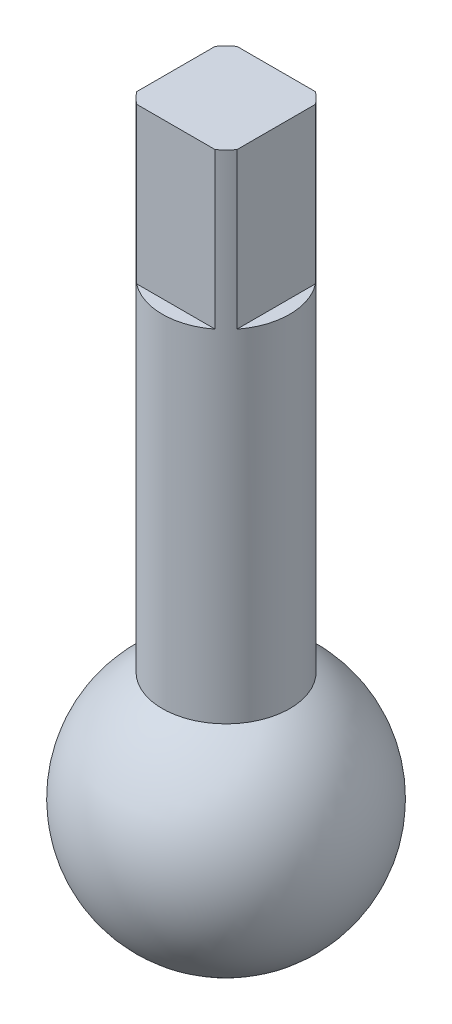
ISO-10303-21;
HEADER;
FILE_DESCRIPTION(('STEP AP214'),'2;1');
FILE_NAME('part.step','',(''),(''),'','','');
FILE_SCHEMA(('AUTOMOTIVE_DESIGN { 1 0 10303 214 1 1 1 1 }'));
ENDSEC;
DATA;
#1=APPLICATION_CONTEXT('core data for automotive mechanical design processes');
#2=APPLICATION_PROTOCOL_DEFINITION('international standard','automotive_design',2000,#1);
#3=PRODUCT_CONTEXT('',#1,'mechanical');
#4=PRODUCT('Part','Part','',(#3));
#5=PRODUCT_RELATED_PRODUCT_CATEGORY('part','',(#4));
#6=PRODUCT_DEFINITION_FORMATION('','',#4);
#7=PRODUCT_DEFINITION_CONTEXT('part definition',#1,'design');
#8=PRODUCT_DEFINITION('design','',#6,#7);
#9=PRODUCT_DEFINITION_SHAPE('','',#8);
#10=(LENGTH_UNIT() NAMED_UNIT(*) SI_UNIT(.MILLI.,.METRE.));
#11=(NAMED_UNIT(*) PLANE_ANGLE_UNIT() SI_UNIT($,.RADIAN.));
#12=(NAMED_UNIT(*) SI_UNIT($,.STERADIAN.) SOLID_ANGLE_UNIT());
#13=UNCERTAINTY_MEASURE_WITH_UNIT(LENGTH_MEASURE(1.E-05),#10,'distance_accuracy_value','');
#14=(GEOMETRIC_REPRESENTATION_CONTEXT(3) GLOBAL_UNCERTAINTY_ASSIGNED_CONTEXT((#13)) GLOBAL_UNIT_ASSIGNED_CONTEXT((#10,
#11,#12)) REPRESENTATION_CONTEXT('',''));
#15=CARTESIAN_POINT('',(0.,0.,0.));
#16=DIRECTION('',(0.,0.,1.));
#17=DIRECTION('',(1.,0.,0.));
#18=AXIS2_PLACEMENT_3D('',#15,#16,#17);
#19=CARTESIAN_POINT('',(0.,90.3,0.));
#20=DIRECTION('',(0.,-1.,0.));
#21=DIRECTION('',(0.,0.,-1.));
#22=AXIS2_PLACEMENT_3D('',#19,#20,#21);
#23=CYLINDRICAL_SURFACE('',#22,12.7);
#24=CARTESIAN_POINT('',(0.,-8.78850096542744,0.));
#25=DIRECTION('',(0.,-1.,0.));
#26=DIRECTION('',(0.,0.,-1.));
#27=AXIS2_PLACEMENT_3D('',#24,#25,#26);
#28=CIRCLE('',#27,12.7);
#29=CARTESIAN_POINT('',(0.,-8.78850096542744,-12.7));
#30=VERTEX_POINT('',#29);
#31=EDGE_CURVE('E11',#30,#30,#28,.T.);
#32=ORIENTED_EDGE('',*,*,#31,.F.);
#33=EDGE_LOOP('',(#32));
#34=FACE_BOUND('',#33,.T.);
#35=DIRECTION('',(0.,1.,0.));
#36=VECTOR('',#35,1.);
#37=CARTESIAN_POINT('',(-7.82879301041993,59.3,10.));
#38=LINE('',#37,#36);
#39=CARTESIAN_POINT('',(-7.82879301041993,59.3,10.));
#40=VERTEX_POINT('',#39);
#41=CARTESIAN_POINT('',(-7.82879301041993,90.3,10.));
#42=VERTEX_POINT('',#41);
#43=EDGE_CURVE('E102',#40,#42,#38,.T.);
#44=ORIENTED_EDGE('',*,*,#43,.T.);
#45=CARTESIAN_POINT('',(0.,90.3,0.));
#46=DIRECTION('',(0.,1.,0.));
#47=DIRECTION('',(0.,0.,1.));
#48=AXIS2_PLACEMENT_3D('',#45,#46,#47);
#49=CIRCLE('',#48,12.7);
#50=CARTESIAN_POINT('',(-10.,90.3,7.82879301041993));
#51=VERTEX_POINT('',#50);
#52=EDGE_CURVE('E130',#51,#42,#49,.T.);
#53=ORIENTED_EDGE('',*,*,#52,.F.);
#54=DIRECTION('',(0.,1.,0.));
#55=VECTOR('',#54,1.);
#56=CARTESIAN_POINT('',(-10.,59.3,7.82879301041993));
#57=LINE('',#56,#55);
#58=CARTESIAN_POINT('',(-10.,59.3,7.82879301041993));
#59=VERTEX_POINT('',#58);
#60=EDGE_CURVE('E57',#59,#51,#57,.T.);
#61=ORIENTED_EDGE('',*,*,#60,.F.);
#62=CARTESIAN_POINT('',(0.,59.3,0.));
#63=DIRECTION('',(0.,1.,0.));
#64=DIRECTION('',(0.,0.,1.));
#65=AXIS2_PLACEMENT_3D('',#62,#63,#64);
#66=CIRCLE('',#65,12.7);
#67=CARTESIAN_POINT('',(-10.,59.3,-7.82879301041993));
#68=VERTEX_POINT('',#67);
#69=EDGE_CURVE('E132',#68,#59,#66,.T.);
#70=ORIENTED_EDGE('',*,*,#69,.F.);
#71=DIRECTION('',(0.,1.,0.));
#72=VECTOR('',#71,1.);
#73=CARTESIAN_POINT('',(-10.,59.3,-7.82879301041993));
#74=LINE('',#73,#72);
#75=CARTESIAN_POINT('',(-10.,90.3,-7.82879301041993));
#76=VERTEX_POINT('',#75);
#77=EDGE_CURVE('E131',#68,#76,#74,.T.);
#78=ORIENTED_EDGE('',*,*,#77,.T.);
#79=CARTESIAN_POINT('',(-7.82879301041993,90.3,-10.));
#80=VERTEX_POINT('',#79);
#81=EDGE_CURVE('E170',#80,#76,#49,.T.);
#82=ORIENTED_EDGE('',*,*,#81,.F.);
#83=DIRECTION('',(0.,1.,0.));
#84=VECTOR('',#83,1.);
#85=CARTESIAN_POINT('',(-7.82879301041993,59.3,-10.));
#86=LINE('',#85,#84);
#87=CARTESIAN_POINT('',(-7.82879301041993,59.3,-10.));
#88=VERTEX_POINT('',#87);
#89=EDGE_CURVE('E61',#88,#80,#86,.T.);
#90=ORIENTED_EDGE('',*,*,#89,.F.);
#91=CARTESIAN_POINT('',(0.,59.3,0.));
#92=DIRECTION('',(0.,1.,0.));
#93=DIRECTION('',(0.,0.,1.));
#94=AXIS2_PLACEMENT_3D('',#91,#92,#93);
#95=CIRCLE('',#94,12.7);
#96=CARTESIAN_POINT('',(7.82879301041993,59.3,-10.));
#97=VERTEX_POINT('',#96);
#98=EDGE_CURVE('E145',#97,#88,#95,.T.);
#99=ORIENTED_EDGE('',*,*,#98,.F.);
#100=DIRECTION('',(0.,1.,0.));
#101=VECTOR('',#100,1.);
#102=CARTESIAN_POINT('',(7.82879301041993,59.3,-10.));
#103=LINE('',#102,#101);
#104=CARTESIAN_POINT('',(7.82879301041993,90.3,-10.));
#105=VERTEX_POINT('',#104);
#106=EDGE_CURVE('E147',#97,#105,#103,.T.);
#107=ORIENTED_EDGE('',*,*,#106,.T.);
#108=CARTESIAN_POINT('',(10.,90.3,-7.82879301041993));
#109=VERTEX_POINT('',#108);
#110=EDGE_CURVE('E165',#109,#105,#49,.T.);
#111=ORIENTED_EDGE('',*,*,#110,.F.);
#112=DIRECTION('',(0.,1.,0.));
#113=VECTOR('',#112,1.);
#114=CARTESIAN_POINT('',(10.,59.3,-7.82879301041993));
#115=LINE('',#114,#113);
#116=CARTESIAN_POINT('',(10.,59.3,-7.82879301041993));
#117=VERTEX_POINT('',#116);
#118=EDGE_CURVE('E149',#117,#109,#115,.T.);
#119=ORIENTED_EDGE('',*,*,#118,.F.);
#120=CARTESIAN_POINT('',(0.,59.3,0.));
#121=DIRECTION('',(0.,1.,0.));
#122=DIRECTION('',(0.,0.,1.));
#123=AXIS2_PLACEMENT_3D('',#120,#121,#122);
#124=CIRCLE('',#123,12.7);
#125=CARTESIAN_POINT('',(10.,59.3,7.82879301041993));
#126=VERTEX_POINT('',#125);
#127=EDGE_CURVE('E154',#126,#117,#124,.T.);
#128=ORIENTED_EDGE('',*,*,#127,.F.);
#129=DIRECTION('',(0.,1.,0.));
#130=VECTOR('',#129,1.);
#131=CARTESIAN_POINT('',(10.,59.3,7.82879301041993));
#132=LINE('',#131,#130);
#133=CARTESIAN_POINT('',(10.,90.3,7.82879301041993));
#134=VERTEX_POINT('',#133);
#135=EDGE_CURVE('E157',#126,#134,#132,.T.);
#136=ORIENTED_EDGE('',*,*,#135,.T.);
#137=CARTESIAN_POINT('',(7.82879301041993,90.3,10.));
#138=VERTEX_POINT('',#137);
#139=EDGE_CURVE('E47',#138,#134,#49,.T.);
#140=ORIENTED_EDGE('',*,*,#139,.F.);
#141=DIRECTION('',(0.,1.,0.));
#142=VECTOR('',#141,1.);
#143=CARTESIAN_POINT('',(7.82879301041993,59.3,10.));
#144=LINE('',#143,#142);
#145=CARTESIAN_POINT('',(7.82879301041993,59.3,10.));
#146=VERTEX_POINT('',#145);
#147=EDGE_CURVE('E116',#146,#138,#144,.T.);
#148=ORIENTED_EDGE('',*,*,#147,.F.);
#149=CARTESIAN_POINT('',(0.,59.3,0.));
#150=DIRECTION('',(0.,1.,0.));
#151=DIRECTION('',(0.,0.,1.));
#152=AXIS2_PLACEMENT_3D('',#149,#150,#151);
#153=CIRCLE('',#152,12.7);
#154=EDGE_CURVE('E120',#40,#146,#153,.T.);
#155=ORIENTED_EDGE('',*,*,#154,.F.);
#156=EDGE_LOOP('',(#44,#53,#61,#70,#78,#82,#90,#99,#107,#111,#119,#128,#136,#140,#148,#155));
#157=FACE_BOUND('',#156,.T.);
#158=ADVANCED_FACE('F41',(#34,#157),#23,.T.);
#159=CARTESIAN_POINT('',(0.,90.3,0.));
#160=DIRECTION('',(0.,1.,0.));
#161=DIRECTION('',(0.,0.,1.));
#162=AXIS2_PLACEMENT_3D('',#159,#160,#161);
#163=PLANE('',#162);
#164=ORIENTED_EDGE('',*,*,#52,.T.);
#165=DIRECTION('',(1.,0.,0.));
#166=VECTOR('',#165,1.);
#167=CARTESIAN_POINT('',(0.,90.3,10.));
#168=LINE('',#167,#166);
#169=EDGE_CURVE('E111',#42,#138,#168,.T.);
#170=ORIENTED_EDGE('',*,*,#169,.T.);
#171=ORIENTED_EDGE('',*,*,#139,.T.);
#172=DIRECTION('',(0.,0.,-1.));
#173=VECTOR('',#172,1.);
#174=CARTESIAN_POINT('',(10.,90.3,0.));
#175=LINE('',#174,#173);
#176=EDGE_CURVE('E151',#134,#109,#175,.T.);
#177=ORIENTED_EDGE('',*,*,#176,.T.);
#178=ORIENTED_EDGE('',*,*,#110,.T.);
#179=DIRECTION('',(-1.,0.,0.));
#180=VECTOR('',#179,1.);
#181=CARTESIAN_POINT('',(0.,90.3,-10.));
#182=LINE('',#181,#180);
#183=EDGE_CURVE('E141',#105,#80,#182,.T.);
#184=ORIENTED_EDGE('',*,*,#183,.T.);
#185=ORIENTED_EDGE('',*,*,#81,.T.);
#186=DIRECTION('',(0.,0.,1.));
#187=VECTOR('',#186,1.);
#188=CARTESIAN_POINT('',(-10.,90.3,0.));
#189=LINE('',#188,#187);
#190=EDGE_CURVE('E135',#76,#51,#189,.T.);
#191=ORIENTED_EDGE('',*,*,#190,.T.);
#192=EDGE_LOOP('',(#164,#170,#171,#177,#178,#184,#185,#191));
#193=FACE_BOUND('',#192,.T.);
#194=ADVANCED_FACE('F167',(#193),#163,.T.);
#195=CARTESIAN_POINT('',(10.,59.3,0.));
#196=DIRECTION('',(1.,0.,0.));
#197=DIRECTION('',(0.,0.,-1.));
#198=AXIS2_PLACEMENT_3D('',#195,#196,#197);
#199=PLANE('',#198);
#200=ORIENTED_EDGE('',*,*,#176,.F.);
#201=ORIENTED_EDGE('',*,*,#135,.F.);
#202=DIRECTION('',(0.,0.,-1.));
#203=VECTOR('',#202,1.);
#204=CARTESIAN_POINT('',(10.,59.3,0.));
#205=LINE('',#204,#203);
#206=EDGE_CURVE('E155',#126,#117,#205,.T.);
#207=ORIENTED_EDGE('',*,*,#206,.T.);
#208=ORIENTED_EDGE('',*,*,#118,.T.);
#209=EDGE_LOOP('',(#200,#201,#207,#208));
#210=FACE_BOUND('',#209,.T.);
#211=ADVANCED_FACE('F186',(#210),#199,.T.);
#212=CARTESIAN_POINT('',(0.,59.3,0.));
#213=DIRECTION('',(0.,1.,0.));
#214=DIRECTION('',(0.,0.,1.));
#215=AXIS2_PLACEMENT_3D('',#212,#213,#214);
#216=PLANE('',#215);
#217=ORIENTED_EDGE('',*,*,#206,.F.);
#218=ORIENTED_EDGE('',*,*,#127,.T.);
#219=EDGE_LOOP('',(#217,#218));
#220=FACE_BOUND('',#219,.T.);
#221=ADVANCED_FACE('F193',(#220),#216,.T.);
#222=CARTESIAN_POINT('',(0.,59.3,-10.));
#223=DIRECTION('',(0.,0.,-1.));
#224=DIRECTION('',(-1.,0.,0.));
#225=AXIS2_PLACEMENT_3D('',#222,#223,#224);
#226=PLANE('',#225);
#227=ORIENTED_EDGE('',*,*,#183,.F.);
#228=ORIENTED_EDGE('',*,*,#106,.F.);
#229=DIRECTION('',(-1.,0.,0.));
#230=VECTOR('',#229,1.);
#231=CARTESIAN_POINT('',(0.,59.3,-10.));
#232=LINE('',#231,#230);
#233=EDGE_CURVE('E139',#97,#88,#232,.T.);
#234=ORIENTED_EDGE('',*,*,#233,.T.);
#235=ORIENTED_EDGE('',*,*,#89,.T.);
#236=EDGE_LOOP('',(#227,#228,#234,#235));
#237=FACE_BOUND('',#236,.T.);
#238=ADVANCED_FACE('F199',(#237),#226,.T.);
#239=CARTESIAN_POINT('',(0.,59.3,0.));
#240=DIRECTION('',(0.,1.,0.));
#241=DIRECTION('',(0.,0.,1.));
#242=AXIS2_PLACEMENT_3D('',#239,#240,#241);
#243=PLANE('',#242);
#244=ORIENTED_EDGE('',*,*,#233,.F.);
#245=ORIENTED_EDGE('',*,*,#98,.T.);
#246=EDGE_LOOP('',(#244,#245));
#247=FACE_BOUND('',#246,.T.);
#248=ADVANCED_FACE('F182',(#247),#243,.T.);
#249=CARTESIAN_POINT('',(-10.,59.3,0.));
#250=DIRECTION('',(-1.,0.,0.));
#251=DIRECTION('',(0.,0.,1.));
#252=AXIS2_PLACEMENT_3D('',#249,#250,#251);
#253=PLANE('',#252);
#254=ORIENTED_EDGE('',*,*,#190,.F.);
#255=ORIENTED_EDGE('',*,*,#77,.F.);
#256=DIRECTION('',(0.,0.,1.));
#257=VECTOR('',#256,1.);
#258=CARTESIAN_POINT('',(-10.,59.3,0.));
#259=LINE('',#258,#257);
#260=EDGE_CURVE('E126',#68,#59,#259,.T.);
#261=ORIENTED_EDGE('',*,*,#260,.T.);
#262=ORIENTED_EDGE('',*,*,#60,.T.);
#263=EDGE_LOOP('',(#254,#255,#261,#262));
#264=FACE_BOUND('',#263,.T.);
#265=ADVANCED_FACE('F172',(#264),#253,.T.);
#266=CARTESIAN_POINT('',(0.,59.3,0.));
#267=DIRECTION('',(0.,1.,0.));
#268=DIRECTION('',(0.,0.,1.));
#269=AXIS2_PLACEMENT_3D('',#266,#267,#268);
#270=PLANE('',#269);
#271=ORIENTED_EDGE('',*,*,#260,.F.);
#272=ORIENTED_EDGE('',*,*,#69,.T.);
#273=EDGE_LOOP('',(#271,#272));
#274=FACE_BOUND('',#273,.T.);
#275=ADVANCED_FACE('F176',(#274),#270,.T.);
#276=CARTESIAN_POINT('',(0.,59.3,10.));
#277=DIRECTION('',(0.,0.,1.));
#278=DIRECTION('',(1.,0.,0.));
#279=AXIS2_PLACEMENT_3D('',#276,#277,#278);
#280=PLANE('',#279);
#281=ORIENTED_EDGE('',*,*,#169,.F.);
#282=ORIENTED_EDGE('',*,*,#43,.F.);
#283=DIRECTION('',(1.,0.,0.));
#284=VECTOR('',#283,1.);
#285=CARTESIAN_POINT('',(0.,59.3,10.));
#286=LINE('',#285,#284);
#287=EDGE_CURVE('E108',#40,#146,#286,.T.);
#288=ORIENTED_EDGE('',*,*,#287,.T.);
#289=ORIENTED_EDGE('',*,*,#147,.T.);
#290=EDGE_LOOP('',(#281,#282,#288,#289));
#291=FACE_BOUND('',#290,.T.);
#292=ADVANCED_FACE('F110',(#291),#280,.T.);
#293=CARTESIAN_POINT('',(0.,59.3,0.));
#294=DIRECTION('',(0.,1.,0.));
#295=DIRECTION('',(0.,0.,1.));
#296=AXIS2_PLACEMENT_3D('',#293,#294,#295);
#297=PLANE('',#296);
#298=ORIENTED_EDGE('',*,*,#287,.F.);
#299=ORIENTED_EDGE('',*,*,#154,.T.);
#300=EDGE_LOOP('',(#298,#299));
#301=FACE_BOUND('',#300,.T.);
#302=ADVANCED_FACE('F119',(#301),#297,.T.);
#303=CARTESIAN_POINT('',(0.,-30.67,0.));
#304=DIRECTION('',(-1.,0.,0.));
#305=DIRECTION('',(0.,1.,0.));
#306=AXIS2_PLACEMENT_3D('',#303,#304,#305);
#307=SPHERICAL_SURFACE('',#306,25.3);
#308=CARTESIAN_POINT('',(0.,-30.67,0.));
#309=DIRECTION('',(0.,-1.,0.));
#310=DIRECTION('',(0.,0.,-1.));
#311=AXIS2_PLACEMENT_3D('',#308,#309,#310);
#312=SPHERICAL_SURFACE('',#311,25.3);
#313=ORIENTED_EDGE('',*,*,#31,.T.);
#314=EDGE_LOOP('',(#313));
#315=FACE_BOUND('',#314,.T.);
#316=ADVANCED_FACE('F43',(#315),#312,.T.);
#317=CLOSED_SHELL('',(#158,#194,#211,#221,#238,#248,#265,#275,#292,#302,#316));
#318=MANIFOLD_SOLID_BREP('B2',#317);
#319=ADVANCED_BREP_SHAPE_REPRESENTATION('',(#18,#318),#14);
#320=SHAPE_DEFINITION_REPRESENTATION(#9,#319);
ENDSEC;
END-ISO-10303-21;
